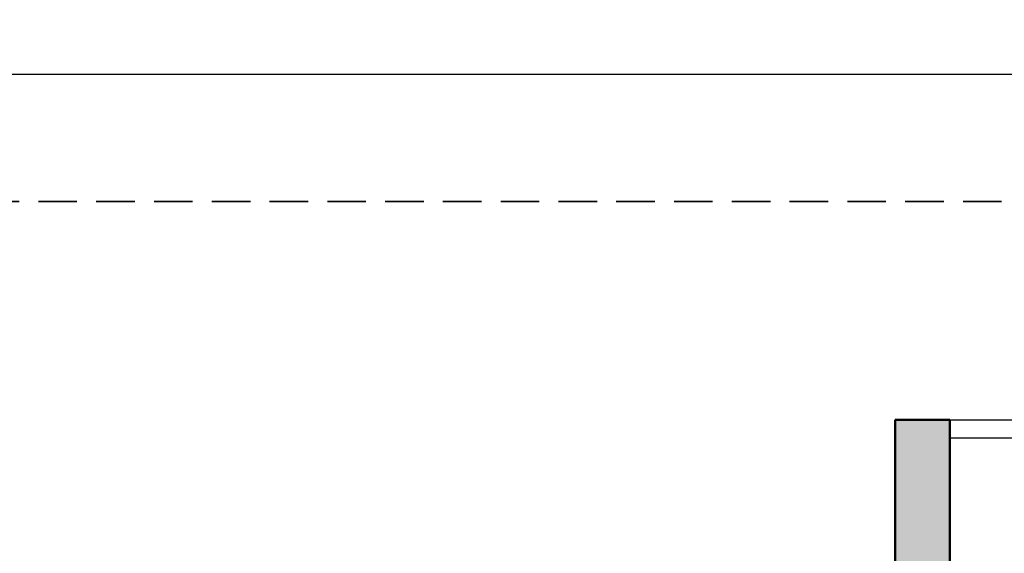
# Model space of a CAD drawing. Units: inches. Extents: x -7 to 1228, y -146 to 1091.
# Tile 81 of 88: x 654 to 816, y 1003 to 1091. Entities that reach past the tile are written whole.
import ezdxf

# ---------------------------------------------------------------- set-up
doc = ezdxf.new("R2010")
doc.units = ezdxf.units.IN
doc.linetypes.add('DASHED2', pattern=[9.525, 6.35, -3.175])
for name, color, linetype, lineweight in [('A-ANNO-DIMS', 2, 'Continuous', 18), ('A-GLAZ', 175, 'Continuous', 25), ('A-WALL', 7, 'Continuous', 50), ('A-WALL-PATT', 251, 'Continuous', 13), ('C-PROP', 1, 'DASHED2', 35)]:
    doc.layers.add(name, color=color, linetype=linetype, lineweight=lineweight)
doc.styles.get("Standard").update_dxf_attribs({"font": 'arial.ttf'})
doc.dimstyles.new('ISO-25', dxfattribs={"dimtxt": 7, "dimasz": 4, "dimexe": 1.25, "dimexo": 0.625, "dimtad": 1, "dimdec": 1, "dimlunit": 3, "dimtxsty": 'Standard', "dimcen": 2.5, "dimadec": 0, "dimazin": 0, "dimtfac": 1, "dimtdec": 1, "dimtmove": 1, "dimatfit": 3, "dimfxl": 1, "dimarcsym": 0})

# ---------------------------------------------------------------- blocks, each defined once
blk = doc.blocks.new('*D11')
at = {"layer": 'A-ANNO-DIMS', "color": 0, "lineweight": -2, "transparency": 16777216}
for p, q in [((0, 1061.62), (0, 1083.25)), ((1187, 1061.62), (1187, 1083.25)), ((4, 1082), (1183, 1082))]:
    blk.add_line(p, q, dxfattribs=at)
at = {"layer": 'A-ANNO-DIMS', "color": 0, "transparency": 16777216}
for points in [[(4, 1082.67), (4, 1081.33), (0, 1082)], [(1183, 1082.67), (1183, 1081.33), (1187, 1082)]]:
    blk.add_solid(points, dxfattribs=at)
at = {"layer": 'Defpoints', "color": 0, "transparency": 16777216}
for p in [(1187, 1082), (0, 1061), (1187, 1061)]:
    blk.add_point(p, dxfattribs=at)
at = {"layer": 'A-ANNO-DIMS', "color": 0, "transparency": 16777216, "insert": (593.5, 1086.2), "char_height": 7, "attachment_point": 5}
blk.add_mtext('98\'-11"', dxfattribs=at)

msp = doc.modelspace()

# ---------------------------------------------------------------- hatches: boundary and pattern name
at = {"layer": 'A-WALL-PATT'}
h = msp.add_hatch(color=256, dxfattribs=at)
h.dxf.hatch_style = 1
h.paths.add_polyline_path([(69, 568), (60, 568), (60, 493), (63.29, 493), (69, 493)])
h.paths.add_polyline_path([(69, 662.41), (60, 662.41), (60, 586), (69, 586)], flags=17)
h.paths.add_polyline_path([(69, 723), (184, 723), (184, 734), (179, 734), (179, 728), (69, 728), (69, 741.62), (60, 741.62), (60, 698.41), (69, 698.41)], flags=17)
h.paths.add_polyline_path([(69, 782), (231, 782), (231, 728), (231, 723), (231, 586), (236, 586), (236, 787), (69, 787), (69, 800.13), (60, 800.13), (60, 765.62), (69, 765.62)])
h.paths.add_polyline_path([(184, 842), (189, 842), (189, 848), (173, 848), (173, 842), (179, 842), (179, 787), (184, 787)])
h.paths.add_polyline_path([(118.22, 69), (69, 69), (69, 60), (118.22, 60)])
h.paths.add_polyline_path([(227, 69), (154.22, 69), (154.22, 60), (227, 60)])
h.paths.add_polyline_path([(236, 60), (232.71, 60), (227, 60), (227, 36), (236, 36)])
h.paths.add_polyline_path([(389, 60), (380, 60), (380, 36), (389, 36)])
h.paths.add_polyline_path([(384, 181), (380, 181), (380, 115), (380, 78), (384, 78)])
h.paths.add_polyline_path([(380, 115), (334.55, 115), (334.55, 109), (380, 109)])
h.paths.add_polyline_path([(274.55, 115), (236, 115), (236, 201), (232.71, 201), (231, 201), (231, 78), (236, 78), (236, 109), (274.55, 109)])
h.paths.add_polyline_path([(69, 123), (60, 123), (60, 78), (69, 78)])
h.paths.add_polyline_path([(69, 201), (60, 201), (60, 159), (69, 159)])
h.paths.add_polyline_path([(143, 219), (69, 219), (69, 213), (143, 213)], flags=17)
h.paths.add_polyline_path([(189, 219), (184, 219), (184, 274), (231, 274), (231, 219), (236, 219), (236, 279), (184, 279), (184, 297), (179, 297), (179, 279), (69, 279), (69, 290.91), (60, 290.91), (60, 262.18), (69, 262.18), (69, 274), (179, 274), (179, 219), (173, 219), (173, 213), (189, 213)])
h.paths.add_polyline_path([(69, 238.18), (60, 238.18), (60, 219), (69, 219)], flags=17)
h.paths.add_polyline_path([(69, 333), (60, 333), (60, 314.91), (69, 314.91), (69, 316.96)])
h.paths.add_polyline_path([(190, 338), (184, 338), (69, 338), (69, 333), (179, 333), (179, 327), (184, 327), (184, 333.02), (190, 333.05)])
h.paths.add_polyline_path([(69, 386.81), (60, 386.81), (60, 351), (69, 351)])
h.paths.add_polyline_path([(69, 475), (60, 475), (60, 422.81), (69, 422.81)])
h.paths.add_polyline_path([(236, 475), (231, 475), (231, 351.24), (236, 351.24)])
h.paths.add_polyline_path([(384, 475), (380, 475), (380, 362), (384, 362)])
h.paths.add_polyline_path([(547, 307), (439, 307), (439, 356), (445, 356), (445, 362), (433, 362), (433, 307), (380, 307), (380, 244), (380, 241), (384, 241), (384, 301), (433, 301), (433, 277), (439, 277), (439, 301), (547, 301)])
h.paths.add_polyline_path([(547, 241), (439, 241), (439, 247), (433, 247), (433, 235), (547, 235)])
h.paths.add_polyline_path([(450, 69), (440.29, 69), (424.89, 69), (389, 69), (389, 60), (450, 60)])
h.paths.add_polyline_path([(547, 69), (486, 69), (486, 60), (547, 60)])
h.paths.add_polyline_path([(556, 148.27), (547, 148.27), (547, 78), (556, 78)])
h.paths.add_polyline_path([(556, 223), (547, 223), (547, 195), (547, 184.27), (556, 184.27)])
h.paths.add_polyline_path([(556, 311.19), (547, 311.19), (547, 273.08), (556, 273.08)])
h.paths.add_polyline_path([(556, 344), (552.71, 344), (547, 344), (547, 335.19), (556, 335.19)])
h.paths.add_polyline_path([(556, 249.08), (547, 249.08), (547, 241), (556, 241)])
h.paths.add_polyline_path([(547, 362), (475, 362), (475, 356), (547, 356)], flags=0)
h.paths.add_polyline_path([(556, 399.62), (547, 399.62), (547, 362), (556, 362)])
h.paths.add_polyline_path([(556, 475), (547, 475), (547, 435.62), (556, 435.62)])
h.paths.add_polyline_path([(547, 493), (389, 493), (389, 487), (547, 487)])
h.paths.add_polyline_path([(380, 493), (278, 493), (278, 487), (380, 487)])
h.paths.add_polyline_path([(227, 493), (69, 493), (69, 487), (227, 487)])
h.paths.add_polyline_path([(643, 122.44), (634, 122.44), (634, 78), (643, 78)])
h.paths.add_polyline_path([(702.5, 69), (692.79, 69), (677.39, 69), (643, 69), (643, 60), (702.5, 60)])
h.paths.add_polyline_path([(798, 69), (738.5, 69), (738.5, 60), (798, 60)])
h.paths.add_polyline_path([(807, 60), (803.71, 60), (798, 60), (798, 36), (807, 36)])
h.paths.add_polyline_path([(807, 109), (846.75, 109), (846.75, 115), (807, 115), (807, 159), (802, 159), (802, 78), (807, 78)])
h.paths.add_polyline_path([(807, 201), (802, 201), (802, 195), (807, 195)])
h.paths.add_polyline_path([(643, 201), (634, 201), (634, 158.44), (643, 158.44)])
h.paths.add_polyline_path([(756, 225), (751, 225), (751, 219), (643, 219), (643, 213), (756, 213)])
h.paths.add_polyline_path([(643, 240.85), (634, 240.85), (634, 219), (643, 219)])
h.paths.add_polyline_path([(643, 274), (643, 288.63), (634, 288.63), (634, 264.85), (643, 264.85)])
h.paths.add_polyline_path([(802, 279), (756, 279), (756, 297), (751, 297), (751, 279), (643, 279), (643, 274), (751, 274), (751, 255), (756, 255), (756, 274), (802, 274)])
h.paths.add_polyline_path([(807, 333), (803.71, 333), (802, 333), (802, 279), (802, 274), (802, 219), (807, 219)])
h.paths.add_polyline_path([(956, 182), (951, 182), (951, 115), (906.75, 115), (906.75, 109), (951, 109), (951, 78), (956, 78)])
h.paths.add_polyline_path([(960, 60), (951, 60), (951, 36), (960, 36)])
h.paths.add_polyline_path([(1021, 69), (1005.78, 69), (960, 69), (960, 60), (1021, 60)])
h.paths.add_polyline_path([(956, 224), (951, 224), (951, 218), (956, 218)])
h.paths.add_polyline_path([(956, 302), (1004, 302), (1004, 278), (1010, 278), (1010, 302), (1118, 302), (1118, 290.81), (1127, 290.81), (1127, 326.97), (1118, 326.97), (1118, 320.97), (1118, 307), (1010, 307), (1010, 356), (1016, 356), (1016, 362), (1004, 362), (1004, 307), (951, 307), (951, 244), (951, 242), (954.29, 242), (956, 242)])
h.paths.add_polyline_path([(643, 333), (634, 333), (634, 312.63), (643, 312.63), (643, 316.96)])
h.paths.add_polyline_path([(756, 338), (643, 338), (643, 333), (751, 333), (751, 327), (756, 327)])
h.paths.add_polyline_path([(643, 388), (634, 388), (634, 351), (643, 351)])
h.paths.add_polyline_path([(807, 357), (802, 357), (802, 351), (807, 351)])
h.paths.add_polyline_path([(807, 475), (802, 475), (802, 393), (807, 393)])
h.paths.add_polyline_path([(643, 475), (634, 475), (634, 424), (643, 424)])
h.paths.add_polyline_path([(798, 493), (643, 493), (643, 487), (798, 487)])
h.paths.add_polyline_path([(634, 493), (556, 493), (556, 487), (634, 487)])
h.paths.add_polyline_path([(813, 493), (807, 493), (807, 487), (813, 487)])
h.paths.add_polyline_path([(951, 493), (849, 493), (849, 487), (951, 487)])
h.paths.add_polyline_path([(956, 484), (951, 484), (951, 374), (956, 374)])
h.paths.add_polyline_path([(1109, 493), (969, 493), (969, 487), (1109, 487)])
h.paths.add_polyline_path([(1127, 484), (1118, 484), (1118, 450.64), (1127, 450.64)])
h.paths.add_polyline_path([(1127, 414.64), (1118, 414.64), (1118, 365), (1127, 365)])
h.paths.add_polyline_path([(1109, 362), (1046, 362), (1046, 356), (1109, 356)], flags=17)
h.paths.add_polyline_path([(1127, 356), (1123.45, 356), (1118, 356), (1118, 350.97), (1127, 350.97)], flags=0)
h.paths.add_polyline_path([(1127, 266.81), (1118, 266.81), (1118, 262.36), (1118, 242), (1127, 242)], flags=17)
h.paths.add_polyline_path([(1118, 242), (1010, 242), (1010, 248), (1004, 248), (1004, 237), (1118, 237)])
h.paths.add_polyline_path([(1127, 224), (1118, 224), (1118, 170), (1127, 170)])
h.paths.add_polyline_path([(1127, 134), (1118, 134), (1118, 78), (1127, 78)])
h.paths.add_polyline_path([(1118, 69), (1057, 69), (1057, 60), (1118, 60)])
h.paths.add_polyline_path([(227, 571.55), (227, 574), (69, 574), (69, 568), (227, 568)])
h.paths.add_polyline_path([(380, 571.55), (380, 574), (278, 574), (278, 568), (380, 568)])
h.paths.add_polyline_path([(242, 574), (236, 574), (236, 568), (242, 568)])
h.paths.add_polyline_path([(547, 571.55), (547, 574), (389, 574), (389, 568), (547, 568)])
h.paths.add_polyline_path([(384, 733), (380, 733), (380, 586), (384, 586)])
h.paths.add_polyline_path([(556, 646), (634, 646), (634, 655), (547, 655), (547, 586), (556, 586)])
h.paths.add_polyline_path([(634, 574), (556, 574), (556, 568), (634, 568)])
h.paths.add_polyline_path([(643, 655), (634, 655), (634, 586), (643, 586)])
h.paths.add_polyline_path([(798, 574), (643, 574), (643, 568), (798, 568)])
h.paths.add_polyline_path([(643, 663.85), (634, 663.85), (634, 655), (643, 655)])
h.paths.add_polyline_path([(556, 676.97), (547, 676.97), (547, 655), (556, 655)])
h.paths.add_polyline_path([(556, 733), (547, 733), (547, 712.97), (556, 712.97)])
h.paths.add_polyline_path([(643, 710), (634, 710), (634, 699.85), (643, 699.85)])
h.paths.add_polyline_path([(807, 668), (802, 668), (802, 586), (807, 586)])
h.paths.add_polyline_path([(951, 574), (849, 574), (849, 568), (951, 568)])
h.paths.add_polyline_path([(956, 691), (951, 691), (951, 577), (956, 577)])
h.paths.add_polyline_path([(1109, 574), (969, 574), (969, 568), (1109, 568)])
h.paths.add_polyline_path([(1127, 643.4), (1118, 643.4), (1118, 577), (1127, 577)])
h.paths.add_polyline_path([(1127, 568), (1123.45, 568), (1118, 568), (1118, 493), (1127, 493)])
h.paths.add_polyline_path([(1127, 733), (1118, 733), (1118, 679.4), (1127, 679.4)])
h.paths.add_polyline_path([(1127, 777.35), (1118, 777.35), (1118, 770.04), (1118, 751), (1127, 751)], flags=17)
h.paths.add_polyline_path([(1118, 751), (1010, 751), (1010, 757), (1004, 757), (1004, 745), (1118, 745)])
h.paths.add_polyline_path([(956, 811), (1004, 811), (1004, 787), (1010, 787), (1010, 811), (1017.87, 811), (1017.87, 811.63, -0.414214), (1018.25, 812), (1031.98, 812, -0.414214), (1032.35, 811.63), (1032.35, 811), (1118, 811), (1118, 801.35), (1127, 801.35), (1127, 834.69), (1118, 834.69), (1118, 830.24), (1118, 817), (1010, 817), (1010, 866), (1016, 866), (1016, 872), (1004, 872), (1004, 817), (956, 817), (956, 866), (951, 866), (951, 751), (954.29, 751), (956, 751)])
h.paths.add_polyline_path([(1118, 872), (1046, 872), (1046, 866), (1118, 866)], flags=17)
h.paths.add_polyline_path([(1127, 924.71), (1118, 924.71), (1118, 884), (1127, 884)])
h.paths.add_polyline_path([(1127, 866), (1123.71, 866), (1118, 866), (1118, 858.69), (1127, 858.69)], flags=17)
h.paths.add_polyline_path([(956, 983), (951, 983), (951, 952), (807, 952), (807, 983), (802, 983), (802, 902), (807, 902), (807, 946), (951, 946), (951, 884), (956, 884)])
h.paths.add_polyline_path([(807, 842), (802, 842), (802, 787), (756, 787), (756, 806), (751, 806), (751, 787), (643, 787), (643, 782), (751, 782), (751, 764), (756, 764), (756, 782), (802, 782), (802, 728), (807, 728)])
h.paths.add_polyline_path([(756, 848), (643, 848), (643, 842), (751, 842), (751, 836), (756, 836)])
h.paths.add_polyline_path([(756, 734), (751, 734), (751, 728), (643, 728), (643, 723), (756, 723)])
h.paths.add_polyline_path([(643, 749.79), (634, 749.79), (634, 728), (637.29, 728), (643, 728)])
h.paths.add_polyline_path([(643, 805.41), (634, 805.41), (634, 773.79), (643, 773.79)])
h.paths.add_polyline_path([(643, 896.66), (634, 896.66), (634, 860), (637.29, 860), (643, 860)])
h.paths.add_polyline_path([(643, 842), (634, 842), (634, 829.41), (643, 829.41)])
h.paths.add_polyline_path([(643, 983), (634, 983), (634, 932.66), (643, 932.66)])
h.paths.add_polyline_path([(1127, 983), (1118, 983), (1118, 960.71), (1127, 960.71)])
h.paths.add_polyline_path([(1118, 1001), (1077.53, 1001), (1077.53, 992), (1118, 992)])
h.paths.add_polyline_path([(1041.53, 1001), (960, 1001), (960, 992), (1041.53, 992)])
h.paths.add_polyline_path([(960, 1025), (951, 1025), (951, 1001), (954.29, 1001), (960, 1001)])
h.paths.add_polyline_path([(807, 1025), (798, 1025), (798, 1001), (807, 1001)])
h.paths.add_polyline_path([(798, 1001), (738.5, 1001), (738.5, 992), (798, 992)])
h.paths.add_polyline_path([(702.5, 1001), (643, 1001), (643, 992), (702.5, 992)])
h.paths.add_polyline_path([(547, 1001), (499.11, 1001), (499.11, 992), (547, 992)])
h.paths.add_polyline_path([(463.11, 1001), (389, 1001), (389, 992), (463.11, 992)])
h.paths.add_polyline_path([(389, 1025), (380, 1025), (380, 1022), (380, 1001), (383.29, 1001), (389, 1001)])
h.paths.add_polyline_path([(236, 1025), (227, 1025), (227, 1001), (236, 1001)])
h.paths.add_polyline_path([(236, 983), (231, 983), (231, 860), (236, 860)])
h.paths.add_polyline_path([(274.55, 952), (236, 952), (236, 946), (274.55, 946)])
h.paths.add_polyline_path([(380, 952), (334.55, 952), (334.55, 946), (380, 946)])
h.paths.add_polyline_path([(384, 983), (380, 983), (380, 884), (383.29, 884), (384, 884)])
h.paths.add_polyline_path([(227, 1001), (155.01, 1001), (155.01, 992), (162.87, 992), (227, 992)])
h.paths.add_polyline_path([(119.01, 1001), (69, 1001), (69, 992), (119.01, 992)])
h.paths.add_polyline_path([(69, 983), (60, 983), (60, 922.99), (69, 922.99)])
h.paths.add_polyline_path([(69, 886.99), (60, 886.99), (60, 860), (63.29, 860), (69, 860)])
h.paths.add_polyline_path([(143, 848), (69, 848), (69, 842), (143, 842)])

# ---------------------------------------------------------------- linework, layer by layer
at = {"layer": 'A-GLAZ'}
for p, q in [((807, 1025), (951, 1025)), ((951, 1022), (807, 1022))]:
    msp.add_line(p, q, dxfattribs=at)
at = {"layer": 'A-WALL'}
for p, q in [((798, 1001), (798, 1025)), ((798, 1025), (807, 1025)), ((807, 1025), (807, 1001))]:
    msp.add_line(p, q, dxfattribs=at)
at = {"layer": 'C-PROP'}
msp.add_line((1187, 1061), (0, 1061), dxfattribs=at)

# ---------------------------------------------------------------- dimensions: what is measured, and where the dimension line sits
at = {"layer": 'A-ANNO-DIMS'}
dim = msp.add_linear_dim(base=(1187, 1082), p1=(0, 1061), p2=(1187, 1061), dimstyle='ISO-25', override={"dimclrd": 0, "dimclre": 0, "dimclrt": 0}, dxfattribs=at)
dim.commit()
dim.dimension.update_dxf_attribs({"geometry": '*D11', "text_midpoint": (593.5, 1086.2)})

doc.saveas('drawing.dxf')
